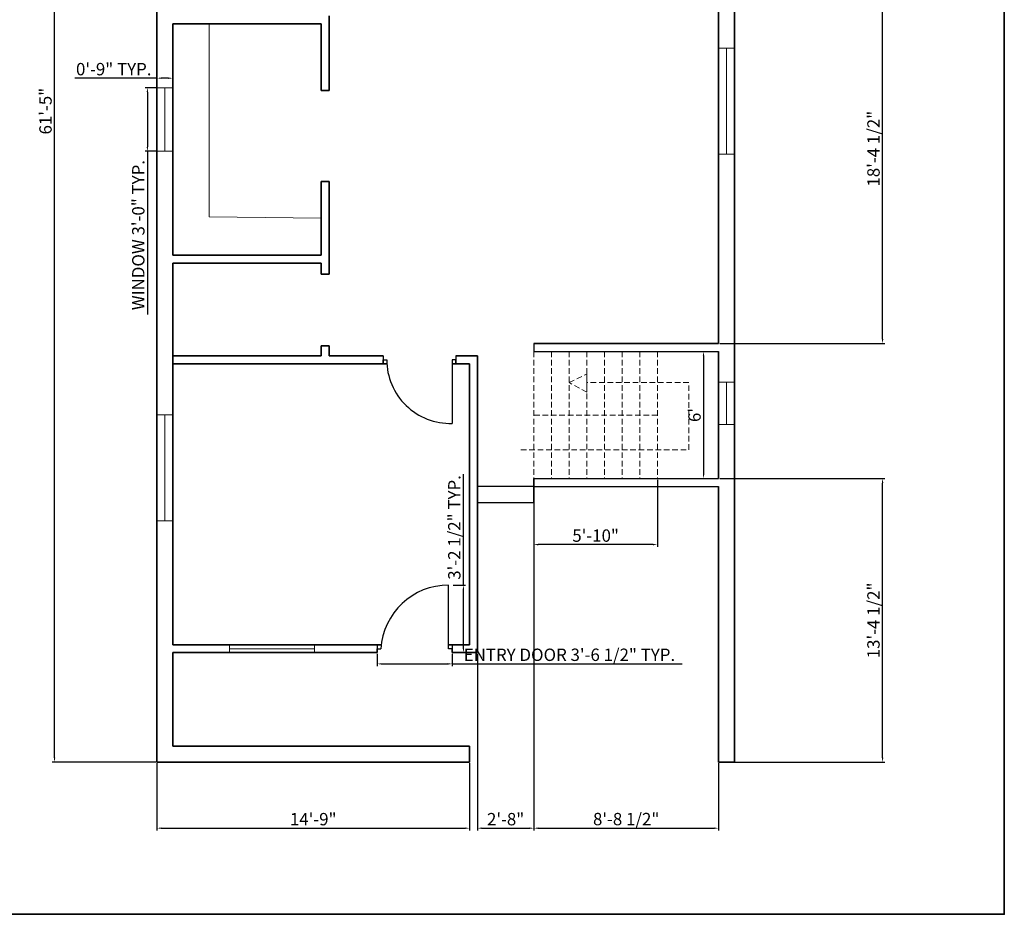
# Model space of a CAD drawing. Units: inches. Extents: x 1863 to 2938, y 1238 to 2492.
# Tile 8 of 12: x 2381 to 2938, y 1253 to 1760. Entities that reach past the tile are written whole.
import ezdxf

# ---------------------------------------------------------------- set-up
doc = ezdxf.new("R2010")
doc.units = ezdxf.units.IN
doc.linetypes.add('HIDDEN2', pattern=[4.7625, 3.175, -1.5875])
for name, color, linetype, lineweight in [('A-ANNO-DIMS', 2, 'Continuous', 18), ('A-ANNO-TTLB', 7, 'Continuous', 35), ('A-DOOR', 3, 'Continuous', 25), ('A-FLOR-FIXT', 9, 'Continuous', 18), ('A-FLOR-STRS', 7, 'Continuous', 25), ('A-FLOR-STRS-HIDN', 253, 'HIDDEN2', 18), ('A-GLAZ', 4, 'Continuous', 18), ('A-WALL', 7, 'Continuous', 35)]:
    doc.layers.add(name, color=color, linetype=linetype, lineweight=lineweight)
doc.styles.get("Standard").update_dxf_attribs({"font": 'arial.ttf'})
doc.dimstyles.new('ISO-25', dxfattribs={"dimtxt": 7, "dimasz": 2.5, "dimexe": 1.25, "dimexo": 0.625, "dimtad": 1, "dimdec": 0, "dimlunit": 3, "dimtxsty": 'Standard', "dimcen": 2.5, "dimadec": 0, "dimazin": 0, "dimtfac": 1, "dimtdec": 0, "dimtmove": 0, "dimatfit": 3, "dimfxl": 1, "dimarcsym": 0})

# ---------------------------------------------------------------- blocks, each defined once
blk = doc.blocks.new('*D4')
at = {"layer": 'A-ANNO-DIMS', "color": 0, "lineweight": -2, "transparency": 16777216}
for p, q in [((2768.11, 1569.56), (2768.11, 1502.56)), ((2768.47, 1572.06), (2769.36, 1572.06)), ((2768.47, 1500.06), (2769.36, 1500.06))]:
    blk.add_line(p, q, dxfattribs=at)
at = {"layer": 'A-ANNO-DIMS', "color": 0, "transparency": 16777216}
for points in [[(2767.69, 1569.56), (2768.53, 1569.56), (2768.11, 1572.06)], [(2767.69, 1502.56), (2768.53, 1502.56), (2768.11, 1500.06)]]:
    blk.add_solid(points, dxfattribs=at)
at = {"layer": 'Defpoints', "color": 0, "transparency": 16777216}
for p in [(2767.85, 1572.06), (2767.85, 1500.06), (2768.11, 1500.06)]:
    blk.add_point(p, dxfattribs=at)
at = {"layer": 'A-ANNO-DIMS', "color": 0, "transparency": 16777216, "insert": (2763.91, 1536.06), "char_height": 7, "attachment_point": 5, "rotation": 90}
blk.add_mtext("6'", dxfattribs=at)
blk = doc.blocks.new('DOOR-36-ENTRY')
for p, q in [((40.4, 2.25), (40.4, 38.25)), ((0, 4.5), (0, 0)), ((0, 0), (0, 2.25)), ((0, 2.25), (2, 2.25)), ((42.4, 2.25), (40.4, 2.25)), ((42.4, 4.5), (42.4, 0)), ((42.4, 0), (42.4, 2.25))]:
    blk.add_line(p, q)
blk.add_arc((40.4, -0.23), 38.48, 90, 176.3006)
blk = doc.blocks.new('DOOR-36-DRAWING')
for p, q in [((0, 38.27), (0, 33.77)), ((0, 33.77), (0, 36.02)), ((0, 36.02), (2, 36.02)), ((41.07, 36.02), (39.07, 36.02)), ((39.07, 36.02), (39.07, 0.02)), ((41.07, 38.27), (41.07, 33.77)), ((41.07, 33.77), (41.07, 36.02))]:
    blk.add_line(p, q)
blk.add_arc((38.02, 36.02), 36.02, 180, 271.6777)
blk = doc.blocks.new('WIN-24')
for p, q in [((0, 24), (9, 24)), ((9, 24), (4.5, 24)), ((4.5, 24), (4.5, 0)), ((4.5, 0), (0, 0)), ((0, 0), (9, 0))]:
    blk.add_line(p, q)
blk = doc.blocks.new('WIN-48')
for p, q in [((0, 4.5), (0, 0)), ((0, 0), (0, 2.25)), ((0, 2.25), (48, 2.25)), ((48, 2.25), (48, 4.5)), ((48, 4.5), (48, 0))]:
    blk.add_line(p, q)
blk = doc.blocks.new('WIN-60')
for p, q in [((0, 60), (9, 60)), ((9, 60), (4.5, 60)), ((4.5, 60), (4.5, 0)), ((4.5, 0), (0, 0)), ((0, 0), (9, 0))]:
    blk.add_line(p, q)
blk = doc.blocks.new('WIN-36')
for p, q in [((0, 36), (9, 36)), ((9, 36), (4.5, 36)), ((4.5, 36), (4.5, 0)), ((4.5, 0), (0, 0)), ((0, 0), (9, 0))]:
    blk.add_line(p, q)
blk = doc.blocks.new('STAIR-FLIGHT-HIDDEN')
for p, q in [((7.32, 72), (7.32, 0)), ((17.32, 72), (17.32, 0)), ((27.32, 72), (27.32, 0)), ((37.32, 72), (37.32, 0)), ((47.32, 72), (47.32, 0)), ((57.32, 72), (57.32, 0)), ((67.32, 72), (67.32, 0)), ((77.32, 72), (77.32, 0)), ((27.32, 54.32), (37.32, 59.21)), ((37.32, 59.21), (37.32, 59.21)), ((37.32, 59.21), (37.32, 48.95)), ((37.32, 48.95), (27.32, 54.32)), ((95.06, 54.32), (37.32, 54.32)), ((95.06, 16.28), (95.06, 54.32)), ((77.32, 36), (7.32, 36)), ((0, 16.28), (95.06, 16.28))]:
    blk.add_line(p, q)
blk = doc.blocks.new('*D32')
at = {"layer": 'A-ANNO-DIMS', "color": 0, "lineweight": -2, "transparency": 16777216}
for p, q in [((2458.01, 1721.32), (2451.98, 1721.32)), ((2453.23, 1718.82), (2453.23, 1687.82)), ((2458.01, 1685.32), (2451.98, 1685.32)), ((2453.23, 1685.32), (2453.23, 1592.99))]:
    blk.add_line(p, q, dxfattribs=at)
at = {"layer": 'A-ANNO-DIMS', "color": 0, "transparency": 16777216}
for points in [[(2452.81, 1718.82), (2453.65, 1718.82), (2453.23, 1721.32)], [(2452.81, 1687.82), (2453.65, 1687.82), (2453.23, 1685.32)]]:
    blk.add_solid(points, dxfattribs=at)
at = {"layer": 'Defpoints', "color": 0, "transparency": 16777216}
for p in [(2458.63, 1721.32), (2453.23, 1685.32), (2458.63, 1685.32)]:
    blk.add_point(p, dxfattribs=at)
at = {"layer": 'A-ANNO-DIMS', "color": 0, "transparency": 16777216, "insert": (2448.98, 1637.9), "char_height": 7, "attachment_point": 5, "rotation": 90}
blk.add_mtext('WINDOW 3\'-0" TYP.', dxfattribs=at)
blk = doc.blocks.new('*D33')
at = {"layer": 'A-ANNO-DIMS', "color": 0, "lineweight": -2, "transparency": 16777216}
for p, q in [((2458.63, 1726.72), (2412.21, 1726.72)), ((2458.63, 1721.94), (2458.63, 1727.97)), ((2465.13, 1726.72), (2461.13, 1726.72)), ((2467.63, 1721.94), (2467.63, 1727.97))]:
    blk.add_line(p, q, dxfattribs=at)
at = {"layer": 'A-ANNO-DIMS', "color": 0, "transparency": 16777216}
for points in [[(2461.13, 1727.13), (2461.13, 1726.3), (2458.63, 1726.72)], [(2465.13, 1727.13), (2465.13, 1726.3), (2467.63, 1726.72)]]:
    blk.add_solid(points, dxfattribs=at)
at = {"layer": 'Defpoints', "color": 0, "transparency": 16777216}
for p in [(2458.63, 1726.72), (2458.63, 1721.32), (2467.63, 1721.32)]:
    blk.add_point(p, dxfattribs=at)
at = {"layer": 'A-ANNO-DIMS', "color": 0, "transparency": 16777216, "insert": (2434.17, 1730.92), "char_height": 7, "attachment_point": 5}
blk.add_mtext('0\'-9" TYP.', dxfattribs=at)
blk = doc.blocks.new('*D54')
at = {"layer": 'A-ANNO-DIMS', "color": 0, "lineweight": -2, "transparency": 16777216}
for p, q in [((2583.4, 1400.94), (2583.4, 1393.95)), ((2625.8, 1400.94), (2625.8, 1393.95)), ((2585.9, 1395.2), (2623.3, 1395.2)), ((2625.8, 1395.2), (2756.07, 1395.2))]:
    blk.add_line(p, q, dxfattribs=at)
at = {"layer": 'A-ANNO-DIMS', "color": 0, "transparency": 16777216}
for points in [[(2585.9, 1395.62), (2585.9, 1394.78), (2583.4, 1395.2)], [(2623.3, 1395.62), (2623.3, 1394.78), (2625.8, 1395.2)]]:
    blk.add_solid(points, dxfattribs=at)
at = {"layer": 'Defpoints', "color": 0, "transparency": 16777216}
for p in [(2583.4, 1401.56), (2625.8, 1401.56), (2625.8, 1395.2)]:
    blk.add_point(p, dxfattribs=at)
at = {"layer": 'A-ANNO-DIMS', "color": 0, "transparency": 16777216, "insert": (2692.19, 1399.45), "char_height": 7, "attachment_point": 5}
blk.add_mtext('ENTRY DOOR 3\'-6 1/2" TYP.', dxfattribs=at)
blk = doc.blocks.new('*D55')
at = {"layer": 'A-ANNO-DIMS', "color": 0, "lineweight": -2, "transparency": 16777216}
for p, q in [((2632.16, 1439.81), (2632.16, 1502.54)), ((2626.42, 1439.81), (2633.41, 1439.81)), ((2632.16, 1404.06), (2632.16, 1437.31)), ((2626.42, 1401.56), (2633.41, 1401.56))]:
    blk.add_line(p, q, dxfattribs=at)
at = {"layer": 'A-ANNO-DIMS', "color": 0, "transparency": 16777216}
for points in [[(2631.74, 1437.31), (2632.58, 1437.31), (2632.16, 1439.81)], [(2631.74, 1404.06), (2632.58, 1404.06), (2632.16, 1401.56)]]:
    blk.add_solid(points, dxfattribs=at)
at = {"layer": 'Defpoints', "color": 0, "transparency": 16777216}
for p in [(2625.8, 1439.81), (2632.16, 1439.81), (2625.8, 1401.56)]:
    blk.add_point(p, dxfattribs=at)
at = {"layer": 'A-ANNO-DIMS', "color": 0, "transparency": 16777216, "insert": (2627.91, 1472.42), "char_height": 7, "attachment_point": 5, "rotation": 90}
blk.add_mtext('3\'-2 1/2" TYP.', dxfattribs=at)
blk = doc.blocks.new('*D60')
at = {"layer": 'A-ANNO-DIMS', "color": 0, "lineweight": -2, "transparency": 16777216}
for p, q in [((2672.01, 1499.44), (2672.01, 1461.46)), ((2742.01, 1499.44), (2742.01, 1461.46)), ((2739.51, 1462.71), (2674.51, 1462.71))]:
    blk.add_line(p, q, dxfattribs=at)
at = {"layer": 'A-ANNO-DIMS', "color": 0, "transparency": 16777216}
for points in [[(2674.51, 1463.13), (2674.51, 1462.3), (2672.01, 1462.71)], [(2739.51, 1463.13), (2739.51, 1462.3), (2742.01, 1462.71)]]:
    blk.add_solid(points, dxfattribs=at)
at = {"layer": 'Defpoints', "color": 0, "transparency": 16777216}
for p in [(2672.01, 1500.06), (2742.01, 1500.06), (2672.01, 1462.71)]:
    blk.add_point(p, dxfattribs=at)
at = {"layer": 'A-ANNO-DIMS', "color": 0, "transparency": 16777216, "insert": (2707.01, 1466.91), "char_height": 7, "attachment_point": 5}
blk.add_mtext('5\'-10"', dxfattribs=at)
blk = doc.blocks.new('*D61')
at = {"layer": 'A-ANNO-DIMS', "color": 0, "lineweight": -2, "transparency": 16777216}
for p, q in [((2458.63, 1338.94), (2458.63, 1300.96)), ((2635.63, 1338.94), (2635.63, 1300.96)), ((2461.13, 1302.21), (2633.13, 1302.21))]:
    blk.add_line(p, q, dxfattribs=at)
at = {"layer": 'A-ANNO-DIMS', "color": 0, "transparency": 16777216}
for points in [[(2461.13, 1302.63), (2461.13, 1301.8), (2458.63, 1302.21)], [(2633.13, 1302.63), (2633.13, 1301.8), (2635.63, 1302.21)]]:
    blk.add_solid(points, dxfattribs=at)
at = {"layer": 'Defpoints', "color": 0, "transparency": 16777216}
for p in [(2458.63, 1339.56), (2635.63, 1339.56), (2635.63, 1302.21)]:
    blk.add_point(p, dxfattribs=at)
at = {"layer": 'A-ANNO-DIMS', "color": 0, "transparency": 16777216, "insert": (2547.13, 1306.41), "char_height": 7, "attachment_point": 5}
blk.add_mtext('14\'-9"', dxfattribs=at)
blk = doc.blocks.new('*D62')
at = {"layer": 'A-ANNO-DIMS', "color": 0, "lineweight": -2, "transparency": 16777216}
for p, q in [((2672.01, 1485.94), (2672.01, 1300.96)), ((2640.13, 1400.94), (2640.13, 1300.96)), ((2642.63, 1302.21), (2669.51, 1302.21))]:
    blk.add_line(p, q, dxfattribs=at)
at = {"layer": 'A-ANNO-DIMS', "color": 0, "transparency": 16777216}
for points in [[(2642.63, 1302.63), (2642.63, 1301.8), (2640.13, 1302.21)], [(2669.51, 1302.63), (2669.51, 1301.8), (2672.01, 1302.21)]]:
    blk.add_solid(points, dxfattribs=at)
at = {"layer": 'Defpoints', "color": 0, "transparency": 16777216}
for p in [(2672.01, 1486.56), (2640.13, 1401.56), (2672.01, 1302.21)]:
    blk.add_point(p, dxfattribs=at)
at = {"layer": 'A-ANNO-DIMS', "color": 0, "transparency": 16777216, "insert": (2656.07, 1306.41), "char_height": 7, "attachment_point": 5}
blk.add_mtext('2\'-8"', dxfattribs=at)
blk = doc.blocks.new('*D63')
at = {"layer": 'A-ANNO-DIMS', "color": 0, "lineweight": -2, "transparency": 16777216}
for p, q in [((2672.01, 1499.44), (2672.01, 1300.96)), ((2776.63, 1338.94), (2776.63, 1300.96)), ((2674.51, 1302.21), (2774.13, 1302.21))]:
    blk.add_line(p, q, dxfattribs=at)
at = {"layer": 'A-ANNO-DIMS', "color": 0, "transparency": 16777216}
for points in [[(2674.51, 1302.63), (2674.51, 1301.8), (2672.01, 1302.21)], [(2774.13, 1302.63), (2774.13, 1301.8), (2776.63, 1302.21)]]:
    blk.add_solid(points, dxfattribs=at)
at = {"layer": 'Defpoints', "color": 0, "transparency": 16777216}
for p in [(2672.01, 1500.06), (2776.63, 1339.56), (2776.63, 1302.21)]:
    blk.add_point(p, dxfattribs=at)
at = {"layer": 'A-ANNO-DIMS', "color": 0, "transparency": 16777216, "insert": (2724.32, 1306.46), "char_height": 7, "attachment_point": 5}
blk.add_mtext('8\'-8 1/2"', dxfattribs=at)
blk = doc.blocks.new('*D65')
at = {"layer": 'A-ANNO-DIMS', "color": 0, "lineweight": -2, "transparency": 16777216}
for p, q in [((2458.01, 2076.56), (2399.39, 2076.56)), ((2400.64, 1342.06), (2400.64, 2074.06)), ((2458.01, 1339.56), (2399.39, 1339.56))]:
    blk.add_line(p, q, dxfattribs=at)
at = {"layer": 'A-ANNO-DIMS', "color": 0, "transparency": 16777216}
for points in [[(2400.22, 2074.06), (2401.06, 2074.06), (2400.64, 2076.56)], [(2400.22, 1342.06), (2401.06, 1342.06), (2400.64, 1339.56)]]:
    blk.add_solid(points, dxfattribs=at)
at = {"layer": 'Defpoints', "color": 0, "transparency": 16777216}
for p in [(2400.64, 2076.56), (2458.63, 2076.56), (2458.63, 1339.56)]:
    blk.add_point(p, dxfattribs=at)
at = {"layer": 'A-ANNO-DIMS', "color": 0, "transparency": 16777216, "insert": (2396.44, 1708.06), "char_height": 7, "attachment_point": 5, "rotation": 90}
blk.add_mtext('61\'-5"', dxfattribs=at)
blk = doc.blocks.new('*D66')
at = {"layer": 'A-ANNO-DIMS', "color": 0, "lineweight": -2, "transparency": 16777216}
for p, q in [((2777.26, 1500.06), (2870.74, 1500.06)), ((2869.49, 1342.06), (2869.49, 1497.56)), ((2777.26, 1339.56), (2870.74, 1339.56))]:
    blk.add_line(p, q, dxfattribs=at)
at = {"layer": 'A-ANNO-DIMS', "color": 0, "transparency": 16777216}
for points in [[(2869.07, 1497.56), (2869.91, 1497.56), (2869.49, 1500.06)], [(2869.07, 1342.06), (2869.91, 1342.06), (2869.49, 1339.56)]]:
    blk.add_solid(points, dxfattribs=at)
at = {"layer": 'Defpoints', "color": 0, "transparency": 16777216}
for p in [(2776.63, 1500.06), (2869.49, 1500.06), (2776.63, 1339.56)]:
    blk.add_point(p, dxfattribs=at)
at = {"layer": 'A-ANNO-DIMS', "color": 0, "transparency": 16777216, "insert": (2865.24, 1419.81), "char_height": 7, "attachment_point": 5, "rotation": 90}
blk.add_mtext('13\'-4 1/2"', dxfattribs=at)
blk = doc.blocks.new('*D67')
at = {"layer": 'A-ANNO-DIMS', "color": 0, "lineweight": -2, "transparency": 16777216}
for p, q in [((2777.26, 1797.06), (2870.74, 1797.06)), ((2869.49, 1579.06), (2869.49, 1794.56)), ((2777.26, 1576.56), (2870.74, 1576.56))]:
    blk.add_line(p, q, dxfattribs=at)
at = {"layer": 'A-ANNO-DIMS', "color": 0, "transparency": 16777216}
for points in [[(2869.07, 1794.56), (2869.91, 1794.56), (2869.49, 1797.06)], [(2869.07, 1579.06), (2869.91, 1579.06), (2869.49, 1576.56)]]:
    blk.add_solid(points, dxfattribs=at)
at = {"layer": 'Defpoints', "color": 0, "transparency": 16777216}
for p in [(2776.63, 1797.06), (2869.49, 1797.06), (2776.63, 1576.56)]:
    blk.add_point(p, dxfattribs=at)
at = {"layer": 'A-ANNO-DIMS', "color": 0, "transparency": 16777216, "insert": (2865.25, 1686.81), "char_height": 7, "attachment_point": 5, "rotation": 90}
blk.add_mtext('18\'-4 1/2"', dxfattribs=at)

msp = doc.modelspace()

# ---------------------------------------------------------------- linework, layer by layer
at = {"layer": 'A-ANNO-TTLB'}
msp.add_lwpolyline([(1863.2, 2492.19), (2938.41, 2492.19), (2938.41, 1253.47), (1863.2, 1253.47)], close=True, dxfattribs=at)
at = {"layer": 'A-FLOR-FIXT'}
for p, q in [((2488.24, 1757.56), (2488.24, 1648.25)), ((2488.24, 1648.25), (2551.63, 1647.42))]:
    msp.add_line(p, q, dxfattribs=at)
at = {"layer": 'A-FLOR-STRS'}
for p, q in [((2672.01, 1576.56), (2672.01, 1572.06)), ((2672.01, 1572.06), (2776.63, 1572.06)), ((2672.01, 1500.06), (2776.63, 1500.06)), ((2672.01, 1495.56), (2672.01, 1500.06)), ((2672.01, 1500.06), (2672.01, 1497.81)), ((2672.01, 1495.56), (2640.13, 1495.56)), ((2640.13, 1495.56), (2640.13, 1486.56)), ((2672.01, 1495.56), (2776.63, 1495.56)), ((2672.01, 1495.56), (2672.01, 1495.56)), ((2672.01, 1486.56), (2672.01, 1495.56)), ((2640.13, 1486.56), (2672.01, 1486.56))]:
    msp.add_line(p, q, dxfattribs=at)
at = {"layer": 'A-WALL'}
for p, q in [((2458.63, 2076.56), (2458.63, 1339.56)), ((2458.63, 2076.56), (2458.63, 1339.56)), ((2785.63, 2076.56), (2785.63, 1495.56)), ((2776.63, 1792.56), (2776.63, 1576.56)), ((2556.13, 1762.06), (2556.13, 1757.56)), ((2467.63, 1757.56), (2467.63, 1626.56)), ((2467.63, 1757.56), (2551.63, 1757.56)), ((2551.63, 1757.56), (2551.63, 1719.81)), ((2556.13, 1757.56), (2556.13, 1719.81)), ((2551.63, 1719.81), (2556.13, 1719.81)), ((2551.63, 1668.29), (2551.63, 1626.56)), ((2551.63, 1668.29), (2556.13, 1668.29)), ((2556.13, 1668.29), (2556.13, 1615.7)), ((2467.63, 1626.56), (2551.63, 1626.56)), ((2467.63, 1622.06), (2467.63, 1406.06)), ((2467.63, 1622.06), (2551.63, 1622.06)), ((2551.63, 1622.06), (2551.63, 1615.7)), ((2551.63, 1615.7), (2556.13, 1615.7)), ((2551.63, 1575.26), (2551.63, 1569.56)), ((2551.63, 1575.26), (2556.13, 1575.26)), ((2556.13, 1575.26), (2556.13, 1569.56)), ((2672.01, 1576.56), (2776.63, 1576.56)), ((2467.63, 1569.56), (2551.63, 1569.56)), ((2586.73, 1569.56), (2556.13, 1569.56)), ((2635.63, 1569.56), (2627.8, 1569.56)), ((2635.63, 1569.56), (2640.13, 1569.56)), ((2640.13, 1569.56), (2640.13, 1495.56)), ((2776.63, 1572.06), (2776.63, 1500.06)), ((2467.63, 1565.06), (2551.63, 1565.06)), ((2551.63, 1565.06), (2556.13, 1565.06)), ((2556.13, 1565.06), (2588.8, 1565.06)), ((2625.8, 1565.06), (2635.63, 1565.06)), ((2635.63, 1565.06), (2635.63, 1406.06)), ((2640.13, 1495.56), (2640.13, 1401.56)), ((2776.63, 1339.56), (2776.63, 1495.56)), ((2785.63, 1495.56), (2785.63, 1339.56)), ((2467.63, 1406.06), (2585.61, 1406.06)), ((2623.8, 1406.06), (2635.63, 1406.06)), ((2467.63, 1401.56), (2467.63, 1348.56)), ((2467.63, 1401.56), (2583.4, 1401.56)), ((2625.8, 1401.56), (2635.63, 1401.56)), ((2640.13, 1401.56), (2635.63, 1401.56)), ((2467.63, 1348.56), (2635.63, 1348.56)), ((2635.63, 1348.56), (2635.63, 1339.56)), ((2458.63, 1339.56), (2635.63, 1339.56)), ((2785.63, 1339.56), (2776.63, 1339.56))]:
    msp.add_line(p, q, dxfattribs=at)

# ---------------------------------------------------------------- block references
at = {"layer": 'A-DOOR'}
for name, p in [('DOOR-36-DRAWING', (2586.73, 1531.3)), ('DOOR-36-ENTRY', (2583.4, 1401.56))]:
    msp.add_blockref(name, p, dxfattribs=at)
at = {"layer": 'A-FLOR-STRS-HIDN'}
msp.add_blockref('STAIR-FLIGHT-HIDDEN', (2664.7, 1500.06), dxfattribs=at)
at = {"layer": 'A-GLAZ'}
for name, p in [('WIN-60', (2776.63, 1683.62)), ('WIN-60', (2458.63, 1476.09)), ('WIN-48', (2499.76, 1401.56))]:
    msp.add_blockref(name, p, dxfattribs=at)
at = {"layer": 'A-GLAZ', "rotation": 180}
for name, p in [('WIN-36', (2467.63, 1721.32)), ('WIN-24', (2785.63, 1554.67))]:
    msp.add_blockref(name, p, dxfattribs=at)

# ---------------------------------------------------------------- dimensions: what is measured, and where the dimension line sits
at = {"layer": 'A-ANNO-DIMS'}
for base, p1, p2, angle, override, picture, middle in [((2400.64, 2076.56), (2458.63, 1339.56), (2458.63, 2076.56), 90, {"dimdec": 1, "dimlfac": 1, "dimrnd": 0, "dimzin": 1, "dimdsep": 46, "dimlunit": 4, "dimfrac": 2}, '*D65', (2396.44, 1708.06)), ((2869.49, 1797.06), (2776.63, 1576.56), (2776.63, 1797.06), 90, {"dimdec": 1, "dimlfac": 1, "dimrnd": 0, "dimzin": 1, "dimdsep": 46, "dimlunit": 4, "dimfrac": 2}, '*D67', (2865.25, 1686.81)), ((2768.11, 1500.06), (2767.85, 1572.06), (2767.85, 1500.06), 90, {"dimclrd": 0, "dimclre": 0, "dimclrt": 0}, '*D4', (2763.91, 1536.06)), ((2672.01, 1462.71), (2742.01, 1500.06), (2672.01, 1500.06), 180, {"dimdec": 1, "dimlfac": 1, "dimrnd": 0, "dimzin": 1, "dimdsep": 46, "dimlunit": 4, "dimfrac": 2}, '*D60', (2707.01, 1466.91)), ((2869.49, 1500.06), (2776.63, 1339.56), (2776.63, 1500.06), 90, {"dimdec": 1, "dimlfac": 1, "dimrnd": 0, "dimzin": 1, "dimdsep": 46, "dimlunit": 4, "dimfrac": 2}, '*D66', (2865.24, 1419.81))]:
    dim = msp.add_linear_dim(base=base, p1=p1, p2=p2, angle=angle, dimstyle='ISO-25', override=override, dxfattribs=at)
    dim.commit()
    dim.dimension.update_dxf_attribs({"geometry": picture, "text_midpoint": middle})
for base, p1, p2, angle, text, picture, middle in [((2458.63, 1726.72), (2467.63, 1721.32), (2458.63, 1721.32), 180, '<> TYP.', '*D33', (2434.17, 1730.92)), ((2453.23, 1685.32), (2458.63, 1721.32), (2458.63, 1685.32), 270, 'WINDOW <> TYP.', '*D32', (2448.98, 1637.9)), ((2632.1600872, 1439.8118837), (2625.79966271, 1401.5618837), (2625.79966271, 1439.8118837), 90, '<> TYP.', '*D55', (2627.91332731, 1472.42426432))]:
    dim = msp.add_linear_dim(base=base, p1=p1, p2=p2, angle=angle, text=text, dimstyle='ISO-25', override={"dimdec": 1, "dimlfac": 1, "dimrnd": 0, "dimzin": 1, "dimdsep": 46, "dimlunit": 4, "dimfrac": 2}, dxfattribs=at)
    dim.commit()
    dim.dimension.update_dxf_attribs({"geometry": picture, "text_midpoint": middle})
for base, p1, p2, picture, middle in [((2776.63, 1302.21), (2672.01, 1500.06), (2776.63, 1339.56), '*D63', (2724.32, 1306.46)), ((2672.01, 1302.21), (2640.13, 1401.56), (2672.01, 1486.56), '*D62', (2656.07, 1306.41)), ((2635.63, 1302.21), (2458.63, 1339.56), (2635.63, 1339.56), '*D61', (2547.13, 1306.41))]:
    dim = msp.add_linear_dim(base=base, p1=p1, p2=p2, dimstyle='ISO-25', override={"dimdec": 1, "dimlfac": 1, "dimrnd": 0, "dimzin": 1, "dimdsep": 46, "dimlunit": 4, "dimfrac": 2}, dxfattribs=at)
    dim.commit()
    dim.dimension.update_dxf_attribs({"geometry": picture, "text_midpoint": middle})
dim = msp.add_linear_dim(base=(2625.8, 1395.2), p1=(2583.4, 1401.56), p2=(2625.8, 1401.56), text='ENTRY DOOR <> TYP.', dimstyle='ISO-25', override={"dimdec": 1, "dimlfac": 1, "dimrnd": 0, "dimzin": 1, "dimdsep": 46, "dimlunit": 4, "dimfrac": 2}, dxfattribs=at)
dim.commit()
dim.dimension.update_dxf_attribs({"geometry": '*D54', "text_midpoint": (2692.19, 1399.45)})

doc.saveas('drawing.dxf')
